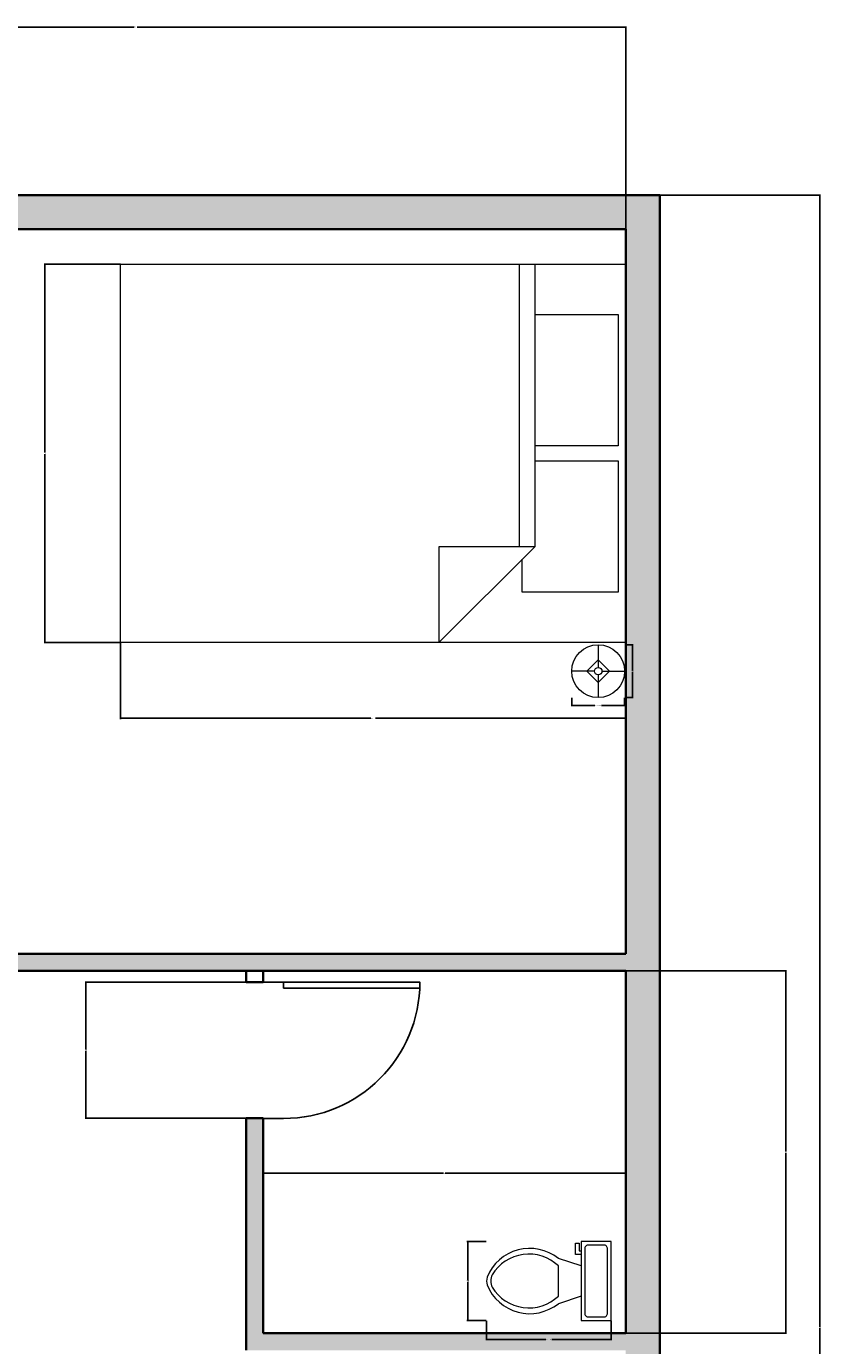
# Model space of a CAD drawing. Units: inches. Extents: x 1563 to 2428, y 777 to 1464.
# Tile 11 of 11: x 2218 to 2428, y 1115 to 1464. Entities that reach past the tile are written whole.
import ezdxf

# ---------------------------------------------------------------- set-up
doc = ezdxf.new("R2010")
doc.units = ezdxf.units.IN
for name, color, linetype, lineweight in [('A-ANNO-DIMS', 2, 'Continuous', 18), ('A-DOOR', 4, 'Continuous', 25), ('A-FLOR-FIXT', 9, 'Continuous', 20), ('A-FURN', 9, 'Continuous', 18), ('A-WALL', 7, 'Continuous', 35), ('A-WALL-PATT', 8, 'Continuous', 13)]:
    doc.layers.add(name, color=color, linetype=linetype, lineweight=lineweight)
doc.styles.get("Standard").update_dxf_attribs({"font": 'arial.ttf'})
doc.dimstyles.get("Standard").update_dxf_attribs({"dimtxt": 0.18, "dimasz": 0.18, "dimexe": 0.18, "dimexo": 0.0625, "dimgap": 0.09, "dimtad": 0, "dimtih": 1, "dimtoh": 1, "dimdec": 4, "dimzin": 0, "dimdsep": 46, "dimtxsty": 'Standard', "dimcen": 0.09, "dimadec": 0, "dimazin": 0, "dimtfac": 1, "dimtdec": 4, "dimtofl": 0, "dimtmove": 0, "dimatfit": 3, "dimfxl": 1, "dimtolj": 1, "dimtzin": 0, "dimarcsym": 0})

# ---------------------------------------------------------------- blocks, each defined once
blk = doc.blocks.new('*U4')
for p, q in [((0, 0), (0, -6)), ((40, 0), (40, -6))]:
    blk.add_line(p, q)
blk.add_lwpolyline([(0, 0), (0, 40), (1.75, 40), (1.75, 0)], close=True)
blk.add_arc((0, 0), 40, 0, 90)
blk = doc.blocks.new('Bed - Queen')
for p, q in [((0, -80.00003), (0, 0)), ((0, 0), (59.99999, 0)), ((59.99999, 0), (59.99999, -80.00003)), ((7.99999, -1.2), (28.79998, -1.2)), ((7.99999, -14.4), (7.99999, -1.2)), ((28.79998, -1.2), (28.79998, -14.4)), ((31.19999, -1.2), (51.99999, -1.2)), ((31.19999, -14.4), (31.19999, -1.2)), ((51.99999, -1.2), (51.99999, -16.4)), ((0, -14.4), (44.8, -14.4)), ((59.99999, -29.6), (44.8, -14.4)), ((44.8, -14.4), (44.8, -29.6)), ((51.99999, -16.4), (46.79936, -16.4)), ((44.8, -16.8), (0, -16.8)), ((44.8, -29.6), (59.99999, -29.6)), ((59.99999, -80.00003), (0, -80.00003))]:
    blk.add_line(p, q)
blk = doc.blocks.new('Lamp - Table')
for p, q in [((0, 7), (0, 1)), ((-1, 0), (-7, 0)), ((0, 3), (-3, 0)), ((-3, 0), (0, -3)), ((3, 0), (0, 3)), ((0, -3), (3, 0)), ((1, 0), (7, 0)), ((0, -1), (0, -7))]:
    blk.add_line(p, q)
for radius in [7, 1]:
    blk.add_circle((0, 0), radius)
blk = doc.blocks.new('Toilet - top')
for p, q in [((9.5, -6), (9.5, -2)), ((-10, -8.5), (-8, -8.5)), ((-10, -9.5), (-10, -8.5)), ((-7, -9.5), (-10, -9.5)), ((-8, -8.5), (-8, -8)), ((-7, -8), (-7, -9.5)), ((-4, -8), (-6, -14)), ((4, -8), (6, -14)), ((4, -14), (-4, -14))]:
    blk.add_line(p, q)
blk.add_lwpolyline([(10.5, -8), (10.5, 0), (-10.5, 0), (-10.5, -8)], close=True)
for points in [[(-9.5, -2), (-9.5, -6)], [(8.5, -1), (-8.5, -1)], [(-8.5, -7), (8.5, -7)]]:
    blk.add_lwpolyline(points)
for centre, radius, start, end in [((-8.62, -1.88), 0.884, 81.8699, 188.1301), ((8.62, -1.88), 0.884, 351.8699, 98.1301), ((-8.62, -6.12), 0.884, 171.8699, 278.1301), ((8.62, -6.12), 0.884, 261.8699, 8.1301), ((3.52, -21.58), 12.17, 141.4691, 247.9714), ((4.2, -21.82), 11.33, 136.3677, 238.9468), ((-3.52, -21.58), 12.17, 292.0284, 38.5307), ((-4.2, -21.82), 11.33, 301.053, 43.6321), ((0, -27.88), 4, 245.7318, 294.2682), ((0, -29), 4, 254.8605, 285.1395)]:
    blk.add_arc(centre, radius, start, end)
blk = doc.blocks.new('*D18')
at = {"layer": 'A-ANNO-DIMS', "color": 0, "lineweight": -2, "transparency": 16777216}
for p, q in [((2362, 1286.15), (2362, 1283.94)), ((2376, 1286.15), (2376, 1283.94)), ((2362.18, 1284.12), (2368.1, 1284.12)), ((2375.82, 1284.12), (2369.9, 1284.12))]:
    blk.add_line(p, q, dxfattribs=at)
at = {"layer": 'A-ANNO-DIMS', "color": 0, "transparency": 16777216}
for points in [[(2362.18, 1284.15), (2362.18, 1284.09), (2362, 1284.12)], [(2375.82, 1284.15), (2375.82, 1284.09), (2376, 1284.12)]]:
    blk.add_solid(points, dxfattribs=at)
at = {"layer": 'Defpoints', "color": 0, "transparency": 16777216}
for p in [(2362, 1286.22), (2376, 1286.22), (2376, 1284.12)]:
    blk.add_point(p, dxfattribs=at)
at = {"layer": 'A-ANNO-DIMS', "color": 0, "transparency": 16777216, "insert": (2369, 1284.12), "char_height": 0.18, "attachment_point": 5}
blk.add_mtext('\\A1;LAMP 14 TYP.', dxfattribs=at)
blk = doc.blocks.new('*D19')
at = {"layer": 'A-ANNO-DIMS', "color": 0, "lineweight": -2, "transparency": 16777216}
for p, q in [((2376.06, 1300.22), (2378.28, 1300.22)), ((2378.1, 1300.04), (2378.1, 1293.4)), ((2378.1, 1286.4), (2378.1, 1293.04)), ((2376.06, 1286.22), (2378.28, 1286.22))]:
    blk.add_line(p, q, dxfattribs=at)
at = {"layer": 'A-ANNO-DIMS', "color": 0, "transparency": 16777216}
for points in [[(2378.07, 1300.04), (2378.13, 1300.04), (2378.1, 1300.22)], [(2378.07, 1286.4), (2378.13, 1286.4), (2378.1, 1286.22)]]:
    blk.add_solid(points, dxfattribs=at)
at = {"layer": 'Defpoints', "color": 0, "transparency": 16777216}
for p in [(2376, 1300.22), (2378.1, 1300.22), (2376, 1286.22)]:
    blk.add_point(p, dxfattribs=at)
at = {"layer": 'A-ANNO-DIMS', "color": 0, "transparency": 16777216, "insert": (2378.1, 1293.22), "char_height": 0.18, "attachment_point": 5}
blk.add_mtext('\\A1;14 TYP.', dxfattribs=at)
blk = doc.blocks.new('*D22')
at = {"layer": 'A-ANNO-DIMS', "color": 0, "lineweight": -2, "transparency": 16777216}
for p, q in [((2242.56, 1300.71), (2242.56, 1280.54)), ((2376.27, 1300.71), (2376.27, 1280.54)), ((2242.74, 1280.72), (2308.84, 1280.72)), ((2376.09, 1280.72), (2310, 1280.72))]:
    blk.add_line(p, q, dxfattribs=at)
at = {"layer": 'A-ANNO-DIMS', "color": 0, "transparency": 16777216}
for points in [[(2242.74, 1280.75), (2242.74, 1280.69), (2242.56, 1280.72)], [(2376.09, 1280.75), (2376.09, 1280.69), (2376.27, 1280.72)]]:
    blk.add_solid(points, dxfattribs=at)
at = {"layer": 'Defpoints', "color": 0, "transparency": 16777216}
for p in [(2242.56, 1300.78), (2376.27, 1300.78), (2376.27, 1280.72)]:
    blk.add_point(p, dxfattribs=at)
at = {"layer": 'A-ANNO-DIMS', "color": 0, "transparency": 16777216, "insert": (2309.42, 1280.72), "char_height": 0.18, "attachment_point": 5}
blk.add_mtext('\\A1;BED 134', dxfattribs=at)
blk = doc.blocks.new('*D23')
at = {"layer": 'A-ANNO-DIMS', "color": 0, "lineweight": -2, "transparency": 16777216}
for p, q in [((2242.5, 1401.06), (2222.33, 1401.06)), ((2222.51, 1400.88), (2222.51, 1351.1)), ((2222.51, 1300.96), (2222.51, 1350.73)), ((2242.5, 1300.78), (2222.33, 1300.78))]:
    blk.add_line(p, q, dxfattribs=at)
at = {"layer": 'A-ANNO-DIMS', "color": 0, "transparency": 16777216}
for points in [[(2222.48, 1400.88), (2222.54, 1400.88), (2222.51, 1401.06)], [(2222.48, 1300.96), (2222.54, 1300.96), (2222.51, 1300.78)]]:
    blk.add_solid(points, dxfattribs=at)
at = {"layer": 'Defpoints', "color": 0, "transparency": 16777216}
for p in [(2242.56, 1401.06), (2222.51, 1300.78), (2242.56, 1300.78)]:
    blk.add_point(p, dxfattribs=at)
at = {"layer": 'A-ANNO-DIMS', "color": 0, "transparency": 16777216, "insert": (2222.51, 1350.92), "char_height": 0.18, "attachment_point": 5}
blk.add_mtext('\\A1;100', dxfattribs=at)
blk = doc.blocks.new('*D36')
at = {"layer": 'A-ANNO-DIMS', "color": 0, "lineweight": -2, "transparency": 16777216}
for p, q in [((2339.4, 1121.1), (2339.4, 1116.03)), ((2372.45, 1121.1), (2372.45, 1116.03)), ((2339.58, 1116.21), (2355.15, 1116.21)), ((2372.27, 1116.21), (2356.7, 1116.21))]:
    blk.add_line(p, q, dxfattribs=at)
at = {"layer": 'A-ANNO-DIMS', "color": 0, "transparency": 16777216}
for points in [[(2339.58, 1116.24), (2339.58, 1116.18), (2339.4, 1116.21)], [(2372.27, 1116.24), (2372.27, 1116.18), (2372.45, 1116.21)]]:
    blk.add_solid(points, dxfattribs=at)
at = {"layer": 'Defpoints', "color": 0, "transparency": 16777216}
for p in [(2339.4, 1121.17), (2372.45, 1121.17), (2372.45, 1116.21)]:
    blk.add_point(p, dxfattribs=at)
at = {"layer": 'A-ANNO-DIMS', "color": 0, "transparency": 16777216, "insert": (2355.92, 1116.21), "char_height": 0.18, "attachment_point": 5}
blk.add_mtext('\\A1;WC 33 TYP.', dxfattribs=at)
blk = doc.blocks.new('*D37')
at = {"layer": 'A-ANNO-DIMS', "color": 0, "lineweight": -2, "transparency": 16777216}
for p, q in [((2339.34, 1142.17), (2334.26, 1142.17)), ((2334.44, 1141.99), (2334.44, 1131.85)), ((2334.44, 1121.35), (2334.44, 1131.49)), ((2339.34, 1121.17), (2334.26, 1121.17))]:
    blk.add_line(p, q, dxfattribs=at)
at = {"layer": 'A-ANNO-DIMS', "color": 0, "transparency": 16777216}
for points in [[(2334.41, 1141.99), (2334.47, 1141.99), (2334.44, 1142.17)], [(2334.41, 1121.35), (2334.47, 1121.35), (2334.44, 1121.17)]]:
    blk.add_solid(points, dxfattribs=at)
at = {"layer": 'Defpoints', "color": 0, "transparency": 16777216}
for p in [(2339.4, 1142.17), (2334.44, 1121.17), (2339.4, 1121.17)]:
    blk.add_point(p, dxfattribs=at)
at = {"layer": 'A-ANNO-DIMS', "color": 0, "transparency": 16777216, "insert": (2334.44, 1131.67), "char_height": 0.18, "attachment_point": 5}
blk.add_mtext('\\A1;21 TYP.', dxfattribs=at)
blk = doc.blocks.new('*D74')
at = {"layer": 'A-ANNO-DIMS', "color": 0, "lineweight": -2, "transparency": 16777216}
for p, q in [((2385.33, 1419.32), (2427.85, 1419.32)), ((2427.67, 1419.14), (2427.67, 1119.51)), ((2427.67, 819.5), (2427.67, 1119.14)), ((2385.33, 819.32), (2427.85, 819.32))]:
    blk.add_line(p, q, dxfattribs=at)
at = {"layer": 'A-ANNO-DIMS', "color": 0, "transparency": 16777216}
for points in [[(2427.64, 1419.14), (2427.7, 1419.14), (2427.67, 1419.32)], [(2427.64, 819.5), (2427.7, 819.5), (2427.67, 819.32)]]:
    blk.add_solid(points, dxfattribs=at)
at = {"layer": 'Defpoints', "color": 0, "transparency": 16777216}
for p in [(2385.27, 1419.32), (2385.27, 819.32), (2427.67, 819.32)]:
    blk.add_point(p, dxfattribs=at)
at = {"layer": 'A-ANNO-DIMS', "color": 0, "transparency": 16777216, "insert": (2427.67, 1119.32), "char_height": 0.18, "attachment_point": 5}
blk.add_mtext('\\A1;600', dxfattribs=at)
blk = doc.blocks.new('*D76')
at = {"layer": 'A-ANNO-DIMS', "color": 0, "lineweight": -2, "transparency": 16777216}
for p, q in [((2116.77, 1410.39), (2116.77, 1464.01)), ((2116.95, 1463.83), (2246.12, 1463.83)), ((2376.09, 1463.83), (2246.92, 1463.83)), ((2376.27, 1410.39), (2376.27, 1464.01))]:
    blk.add_line(p, q, dxfattribs=at)
at = {"layer": 'A-ANNO-DIMS', "color": 0, "transparency": 16777216}
for points in [[(2116.95, 1463.86), (2116.95, 1463.8), (2116.77, 1463.83)], [(2376.09, 1463.86), (2376.09, 1463.8), (2376.27, 1463.83)]]:
    blk.add_solid(points, dxfattribs=at)
at = {"layer": 'Defpoints', "color": 0, "transparency": 16777216}
for p in [(2376.27, 1463.83), (2116.77, 1410.32), (2376.27, 1410.32)]:
    blk.add_point(p, dxfattribs=at)
at = {"layer": 'A-ANNO-DIMS', "color": 0, "transparency": 16777216, "insert": (2246.52, 1463.83), "char_height": 0.18, "attachment_point": 5}
blk.add_mtext('\\A1;259.5', dxfattribs=at)
blk = doc.blocks.new('*D81')
at = {"layer": 'A-ANNO-DIMS', "color": 0, "lineweight": -2, "transparency": 16777216}
for p, q in [((2280.27, 1117.89), (2280.27, 1160.4)), ((2280.45, 1160.22), (2328.05, 1160.22)), ((2376.09, 1160.22), (2328.49, 1160.22)), ((2376.27, 1117.89), (2376.27, 1160.4))]:
    blk.add_line(p, q, dxfattribs=at)
at = {"layer": 'A-ANNO-DIMS', "color": 0, "transparency": 16777216}
for points in [[(2280.45, 1160.25), (2280.45, 1160.19), (2280.27, 1160.22)], [(2376.09, 1160.25), (2376.09, 1160.19), (2376.27, 1160.22)]]:
    blk.add_solid(points, dxfattribs=at)
at = {"layer": 'Defpoints', "color": 0, "transparency": 16777216}
for p in [(2376.27, 1160.22), (2280.27, 1117.82), (2376.27, 1117.82)]:
    blk.add_point(p, dxfattribs=at)
at = {"layer": 'A-ANNO-DIMS', "color": 0, "transparency": 16777216, "insert": (2328.27, 1160.22), "char_height": 0.18, "attachment_point": 5}
blk.add_mtext('\\A1;96', dxfattribs=at)
blk = doc.blocks.new('*D82')
at = {"layer": 'A-ANNO-DIMS', "color": 0, "lineweight": -2, "transparency": 16777216}
for p, q in [((2376.33, 1213.82), (2418.85, 1213.82)), ((2418.67, 1213.64), (2418.67, 1166.01)), ((2418.67, 1118), (2418.67, 1165.64)), ((2376.33, 1117.82), (2418.85, 1117.82))]:
    blk.add_line(p, q, dxfattribs=at)
at = {"layer": 'A-ANNO-DIMS', "color": 0, "transparency": 16777216}
for points in [[(2418.64, 1213.64), (2418.7, 1213.64), (2418.67, 1213.82)], [(2418.64, 1118), (2418.7, 1118), (2418.67, 1117.82)]]:
    blk.add_solid(points, dxfattribs=at)
at = {"layer": 'Defpoints', "color": 0, "transparency": 16777216}
for p in [(2376.27, 1213.82), (2376.27, 1117.82), (2418.67, 1117.82)]:
    blk.add_point(p, dxfattribs=at)
at = {"layer": 'A-ANNO-DIMS', "color": 0, "transparency": 16777216, "insert": (2418.67, 1165.82), "char_height": 0.18, "attachment_point": 5}
blk.add_mtext('\\A1;96', dxfattribs=at)
blk = doc.blocks.new('*D89')
at = {"layer": 'A-ANNO-DIMS', "color": 0, "lineweight": -2, "transparency": 16777216}
for p, q in [((2275.71, 1210.82), (2233.19, 1210.82)), ((2233.37, 1210.64), (2233.37, 1193.01)), ((2233.37, 1175), (2233.37, 1192.64)), ((2275.71, 1174.82), (2233.19, 1174.82))]:
    blk.add_line(p, q, dxfattribs=at)
at = {"layer": 'A-ANNO-DIMS', "color": 0, "transparency": 16777216}
for points in [[(2233.34, 1210.64), (2233.4, 1210.64), (2233.37, 1210.82)], [(2233.34, 1175), (2233.4, 1175), (2233.37, 1174.82)]]:
    blk.add_solid(points, dxfattribs=at)
at = {"layer": 'Defpoints', "color": 0, "transparency": 16777216}
for p in [(2233.37, 1210.82), (2275.77, 1210.82), (2275.77, 1174.82)]:
    blk.add_point(p, dxfattribs=at)
at = {"layer": 'A-ANNO-DIMS', "color": 0, "transparency": 16777216, "insert": (2233.37, 1192.82), "char_height": 0.18, "attachment_point": 5}
blk.add_mtext('\\A1;36', dxfattribs=at)

msp = doc.modelspace()

# ---------------------------------------------------------------- hatches: boundary and pattern name
at = {"layer": 'A-WALL-PATT'}
h = msp.add_hatch(color=256, dxfattribs=at)
h.dxf.hatch_style = 1
h.paths.add_polyline_path([(2385.27, 1419.324), (2025.27, 1419.324), (2025.27, 819.324), (2385.27, 819.324)])
h.paths.add_polyline_path([(2034.27, 1410.324), (2112.27, 1410.324), (2112.27, 1257.324), (2116.77, 1257.324), (2116.77, 1410.324), (2376.27, 1410.324), (2376.27, 1218.324), (2158.77, 1218.324), (2158.77, 1213.824), (2376.27, 1213.824), (2376.27, 1117.824), (2280.27, 1117.824), (2280.27, 1174.824), (2275.77, 1174.824), (2275.77, 1113.324), (2376.27, 1113.324), (2376.27, 828.324), (2214.27, 828.324), (2214.27, 1039.824), (2211.27, 1039.824), (2211.27, 828.324), (2034.27, 828.324), (2034.27, 1039.824), (2172.27, 1039.824), (2172.27, 1044.324), (2034.27, 1044.324), (2034.27, 1136.044, -0.0910221), (2034.27, 1152.131), (2034.27, 1213.824), (2116.77, 1213.824), (2116.77, 1218.324), (2034.27, 1218.324)], flags=16)
h.paths.add_polyline_path([(2106.854, 1222.904), (2106.854, 1221.324), (2070.749, 1221.324), (2070.749, 1222.904)], flags=0)
h.paths.add_polyline_path([(2112.405, 1204.123), (2112.405, 1184.897), (2107.968, 1184.897), (2107.968, 1186.049), (2054.728, 1186.049), (2054.728, 1184.897), (2050.292, 1184.897), (2050.292, 1204.123, -0.1904762)], flags=0)
h.paths.add_polyline_path([(2090.222, 1205.162), (2090.222, 1200.143), (2072.475, 1200.143), (2072.475, 1205.162, -0.0496282)], flags=0)
h.paths.add_polyline_path([(2154.296, 1259.846), (2155.876, 1259.846), (2155.876, 1223.74), (2154.296, 1223.74)], flags=0)
h.paths.add_polyline_path([(2057.091, 1161.316), (2057.976, 1125.833), (2042.473, 1125.447, -0.2279232), (2041.588, 1160.929)], flags=0)
h.paths.add_polyline_path([(2070.302, 1156.728), (2114.669, 1156.728), (2114.669, 1134.544), (2070.302, 1134.544)], flags=0)
h.paths.add_polyline_path([(2098.463, 1153.659), (2098.693, 1153.693), (2098.873, 1153.74), (2099.01, 1153.799), (2099.116, 1153.868), (2099.197, 1153.947), (2099.257, 1154.032), (2099.297, 1154.124), (2099.319, 1154.22), (2099.325, 1154.317), (2099.317, 1154.416), (2099.296, 1154.513), (2099.264, 1154.608), (2099.223, 1154.698), (2099.175, 1154.784), (2099.152, 1154.822), (2099.024, 1155.024), (2098.98, 1155.1), (2098.886, 1155.294), (2098.952, 1155.577), (2099.204, 1155.752), (2099.49, 1155.809), (2099.811, 1155.818), (2100.249, 1155.79), (2100.399, 1155.774), (2100.143, 1155.797), (2099.922, 1155.811), (2099.732, 1155.816), (2099.57, 1155.811), (2099.432, 1155.797), (2099.315, 1155.774), (2099.215, 1155.742), (2099.129, 1155.7), (2099.057, 1155.651), (2099, 1155.594), (2098.956, 1155.532), (2098.926, 1155.465), (2098.91, 1155.395), (2098.907, 1155.322), (2098.919, 1155.249), (2098.944, 1155.175), (2098.98, 1155.1), (2099.024, 1155.024), (2099.073, 1154.947), (2099.124, 1154.867), (2099.239, 1154.68), (2099.35, 1154.353), (2099.273, 1154.02), (2099.025, 1153.78), (2098.599, 1153.668)], flags=0)
h.paths.add_polyline_path([(2102.466, 1148.582), (2102.722, 1148.584), (2102.944, 1148.598), (2103.134, 1148.624), (2103.296, 1148.662), (2103.434, 1148.711), (2103.551, 1148.771), (2103.651, 1148.84), (2103.737, 1148.919), (2103.808, 1149.01), (2103.864, 1149.116), (2103.904, 1149.241), (2103.928, 1149.386), (2103.936, 1149.554), (2103.926, 1149.749), (2103.898, 1149.974), (2103.852, 1150.229), (2103.791, 1150.508), (2103.719, 1150.804), (2103.639, 1151.108), (2103.554, 1151.411), (2103.468, 1151.707), (2103.384, 1151.986), (2103.306, 1152.242), (2103.192, 1152.613), (2103.109, 1152.925), (2103.073, 1153.241), (2103.204, 1153.522), (2103.537, 1153.75), (2103.928, 1153.83), (2104.287, 1153.815), (2104.697, 1153.701), (2104.827, 1153.641), (2104.593, 1153.73), (2104.384, 1153.788), (2104.194, 1153.819), (2104.014, 1153.826), (2103.845, 1153.813), (2103.688, 1153.781), (2103.546, 1153.733), (2103.421, 1153.671), (2103.313, 1153.597), (2103.225, 1153.514), (2103.158, 1153.425), (2103.114, 1153.329), (2103.091, 1153.226), (2103.088, 1153.111), (2103.103, 1152.981), (2103.134, 1152.832), (2103.179, 1152.662), (2103.237, 1152.466), (2103.306, 1152.242), (2103.384, 1151.986), (2103.468, 1151.707), (2103.554, 1151.411), (2103.639, 1151.108), (2103.719, 1150.804), (2103.831, 1150.346), (2103.921, 1149.846), (2103.94, 1149.459), (2103.881, 1149.105), (2103.667, 1148.829), (2103.373, 1148.68), (2103.05, 1148.605), (2102.609, 1148.576)], flags=0)
h.paths.add_polyline_path([(2105.563, 1146.7), (2105.82, 1146.77), (2106.045, 1146.848), (2106.242, 1146.934), (2106.417, 1147.025), (2106.572, 1147.121), (2106.714, 1147.219), (2106.846, 1147.317), (2107.065, 1147.484), (2107.307, 1147.648), (2107.597, 1147.802), (2107.932, 1147.921), (2108.322, 1147.996), (2108.777, 1148.019), (2109.297, 1147.991), (2109.852, 1147.914), (2110.415, 1147.796), (2110.559, 1147.756), (2110.278, 1147.825), (2109.995, 1147.884), (2109.715, 1147.933), (2109.438, 1147.971), (2109.169, 1147.998), (2108.91, 1148.012), (2108.664, 1148.014), (2108.433, 1148.002), (2108.22, 1147.977), (2108.024, 1147.939), (2107.843, 1147.889), (2107.675, 1147.83), (2107.519, 1147.76), (2107.372, 1147.683), (2107.234, 1147.599), (2107.102, 1147.509), (2106.974, 1147.415), (2106.747, 1147.242), (2106.488, 1147.063), (2106.146, 1146.883), (2105.705, 1146.729)], flags=0)
h.paths.add_polyline_path([(2114.376, 1144.033), (2114.426, 1144.021), (2114.436, 1144.02), (2114.305, 1144.051)], flags=0)
h.paths.add_polyline_path([(2242.564, 1401.056), (2376.27, 1401.056), (2376.27, 1300.776), (2242.564, 1300.776)], flags=0)
h.paths.add_polyline_path([(2326.799, 1326.18), (2352.203, 1326.18), (2352.203, 1387.685), (2374.265, 1387.685), (2374.265, 1352.922), (2352.203, 1352.922), (2352.203, 1348.91), (2374.265, 1348.91), (2374.265, 1314.147), (2348.86, 1314.147), (2348.86, 1322.838), (2326.799, 1300.776)], flags=0)
h.paths.add_polyline_path([(2313.978, 1083.124), (2342.025, 1083.124), (2370.073, 1083.124), (2370.073, 977.167), (2342.025, 977.167), (2313.978, 977.167)], flags=0)
h.paths.add_polyline_path([(1834.605, 1034.428), (1914.224, 1034.428), (1914.224, 1038.928), (1614.105, 1038.928), (1614.105, 1034.428), (1830.105, 1034.428), (1830.105, 830.428), (1834.605, 830.428)])

# ---------------------------------------------------------------- linework, layer by layer
at = {"layer": 'A-WALL'}
for p, q in [((2116.77, 1410.324), (2376.27, 1410.324)), ((2376.27, 1410.324), (2376.27, 1218.324)), ((2155.77, 1218.324), (2376.27, 1218.324)), ((2155.77, 1213.824), (2376.27, 1213.824)), ((2275.77, 1213.824), (2275.77, 1210.824)), ((2280.27, 1213.824), (2280.27, 1210.824)), ((2376.27, 1213.824), (2376.27, 1117.824)), ((2275.77, 1210.824), (2280.27, 1210.824)), ((2275.77, 1174.824), (2280.27, 1174.824)), ((2275.77, 1174.824), (2275.77, 1113.324)), ((2280.27, 1174.824), (2280.27, 1117.824)), ((2280.27, 1117.824), (2376.27, 1117.824))]:
    msp.add_line(p, q, dxfattribs=at)
msp.add_lwpolyline([(2025.27, 1419.324), (2385.27, 1419.324), (2385.27, 819.324), (2025.27, 819.324)], close=True, dxfattribs=at)

# ---------------------------------------------------------------- block references
at = {"layer": 'A-DOOR', "xscale": 0.9026413098436022, "yscale": 0.9026413098436022, "zscale": 0.9026413098436022, "rotation": 270}
msp.add_blockref('*U4', (2285.686, 1210.824), dxfattribs=at)
at = {"layer": 'A-FLOR-FIXT', "rotation": 270}
msp.add_blockref('Toilet - top', (2372.447, 1131.667), dxfattribs=at)
at = {"layer": 'A-FURN', "xscale": 1.671329360166141, "yscale": 1.671329360166141, "zscale": 1.671329360166141, "rotation": 270}
msp.add_blockref('Bed - Queen', (2376.27, 1401.056), dxfattribs=at)
at = {"layer": 'A-FURN'}
msp.add_blockref('Lamp - Table', (2369, 1293.216), dxfattribs=at)

# ---------------------------------------------------------------- dimensions: what is measured, and where the dimension line sits
at = {"layer": 'A-ANNO-DIMS'}
for base, p1, p2, override, picture, middle in [((2376.27, 1463.828), (2116.77, 1410.324), (2376.27, 1410.324), {"dimdec": 1, "dimlfac": 1, "dimrnd": 0, "dimzin": 0, "dimdsep": 46, "dimlunit": 2}, '*D76', (2246.52, 1463.828)), ((2376.27, 1160.224), (2280.27, 1117.824), (2376.27, 1117.824), {"dimdec": 0, "dimlfac": 1, "dimrnd": 0, "dimzin": 0, "dimdsep": 46, "dimlunit": 2}, '*D81', (2328.27, 1160.224))]:
    dim = msp.add_linear_dim(base=base, p1=p1, p2=p2, dimstyle='Standard', override=override, dxfattribs=at)
    dim.commit()
    dim.dimension.update_dxf_attribs({"geometry": picture, "text_midpoint": middle})
for base, p1, p2, angle, picture, middle in [((2427.67, 819.324), (2385.27, 1419.324), (2385.27, 819.324), 270, '*D74', (2427.67, 1119.324)), ((2222.508, 1300.776), (2242.564, 1401.056), (2242.564, 1300.776), 270, '*D23', (2222.508, 1350.916)), ((2418.67, 1117.824), (2376.27, 1213.824), (2376.27, 1117.824), 270, '*D82', (2418.67, 1165.824)), ((2233.37, 1210.824), (2275.77, 1174.824), (2275.77, 1210.824), 90, '*D89', (2233.37, 1192.824))]:
    dim = msp.add_linear_dim(base=base, p1=p1, p2=p2, angle=angle, dimstyle='Standard', override={"dimdec": 0, "dimlfac": 1, "dimrnd": 0, "dimzin": 0, "dimdsep": 46, "dimlunit": 2}, dxfattribs=at)
    dim.commit()
    dim.dimension.update_dxf_attribs({"geometry": picture, "text_midpoint": middle})
for base, p1, p2, text, picture, middle in [((2376.27, 1280.72), (2242.564, 1300.776), (2376.27, 1300.776), 'BED <>', '*D22', (2309.417, 1280.72)), ((2376, 1284.116), (2362, 1286.216), (2376, 1286.216), 'LAMP <> TYP.', '*D18', (2369, 1284.116)), ((2372.447, 1116.21), (2339.401, 1121.167), (2372.447, 1121.167), 'WC <> TYP.', '*D36', (2355.924, 1116.21))]:
    dim = msp.add_linear_dim(base=base, p1=p1, p2=p2, text=text, dimstyle='Standard', override={"dimdec": 0, "dimlfac": 1, "dimrnd": 0, "dimzin": 0, "dimdsep": 46, "dimlunit": 2}, dxfattribs=at)
    dim.commit()
    dim.dimension.update_dxf_attribs({"geometry": picture, "text_midpoint": middle})
for base, p1, p2, angle, picture, middle in [((2378.1, 1300.216), (2376, 1286.216), (2376, 1300.216), 90, '*D19', (2378.1, 1293.216)), ((2334.444, 1121.167), (2339.401, 1142.167), (2339.401, 1121.167), 270, '*D37', (2334.444, 1131.667))]:
    dim = msp.add_linear_dim(base=base, p1=p1, p2=p2, angle=angle, text='<> TYP.', dimstyle='Standard', override={"dimdec": 0, "dimlfac": 1, "dimrnd": 0, "dimzin": 0, "dimdsep": 46, "dimlunit": 2}, dxfattribs=at)
    dim.commit()
    dim.dimension.update_dxf_attribs({"geometry": picture, "text_midpoint": middle})

doc.saveas('drawing.dxf')
